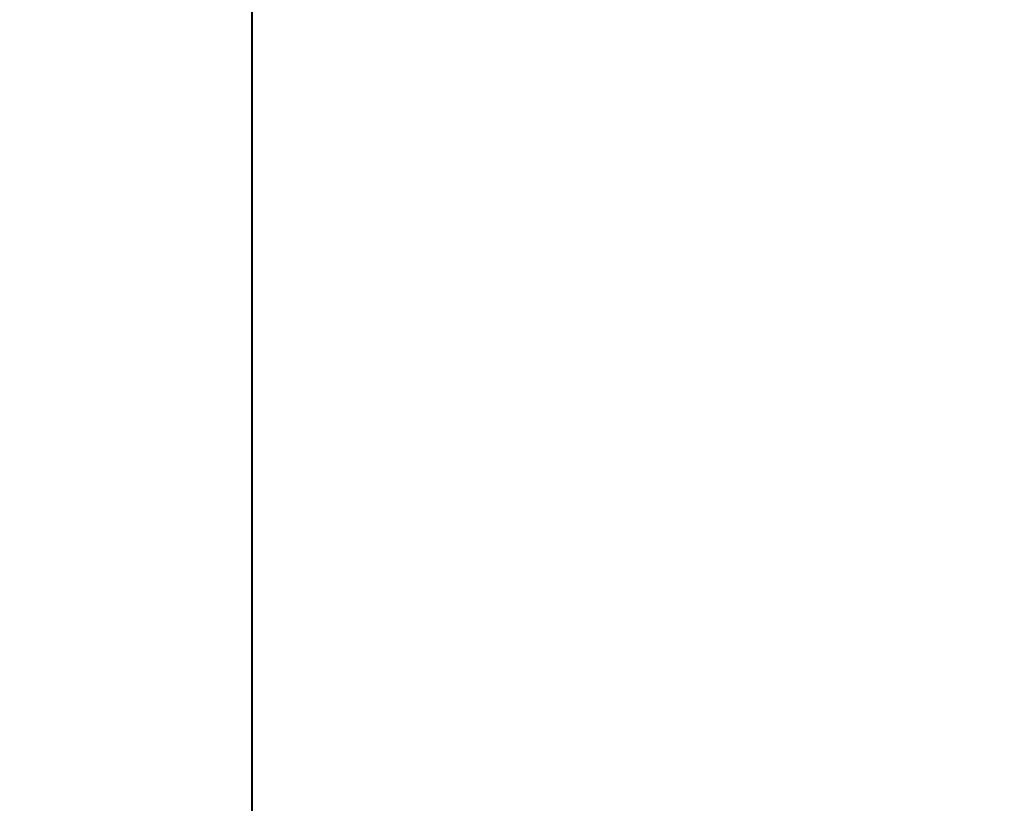
# Model space of a CAD drawing. Units: inches. Extents: x 459864 to 460310, y 324185 to 324787.
# Tile 99 of 112: x 460246.614 to 460248.739, y 324285.121 to 324286.812. Entities that reach past the tile are written whole.
import ezdxf

# ---------------------------------------------------------------- set-up
doc = ezdxf.new("R2010")
doc.units = ezdxf.units.IN
doc.layers.add('A-ANNO-DIMS', color=2, linetype='Continuous', lineweight=18)
doc.layers.add('A-WALL', color=7, linetype='Continuous', lineweight=40)
doc.styles.get("Standard").update_dxf_attribs({"font": 'arial.ttf'})
doc.dimstyles.new('ISO-25', dxfattribs={"dimtxt": 6, "dimasz": 2.5, "dimexe": 1.25, "dimexo": 0.625, "dimtad": 1, "dimdec": 1, "dimlunit": 3, "dimtxsty": 'Standard', "dimcen": 2.5, "dimadec": 0, "dimazin": 0, "dimtfac": 1, "dimtdec": 1, "dimtmove": 0, "dimatfit": 3, "dimfxl": 1, "dimarcsym": 0})

# ---------------------------------------------------------------- blocks, each defined once
blk = doc.blocks.new('*D21')
at = {"layer": 'A-ANNO-DIMS', "color": 0, "lineweight": -2, "transparency": 16777216}
for p, q in [((460247.7399, 324715.4832), (460309.5804, 324715.4832)), ((460308.3304, 324712.9832), (460308.3304, 324285.9832)), ((460247.7399, 324283.4832), (460309.5804, 324283.4832))]:
    blk.add_line(p, q, dxfattribs=at)
at = {"layer": 'A-ANNO-DIMS', "color": 0, "transparency": 16777216}
for points in [[(460307.9137, 324712.9832), (460308.747, 324712.9832), (460308.3304, 324715.4832)], [(460307.9137, 324285.9832), (460308.747, 324285.9832), (460308.3304, 324283.4832)]]:
    blk.add_solid(points, dxfattribs=at)
at = {"layer": 'Defpoints', "color": 0, "transparency": 16777216}
for p in [(460247.1149, 324715.4832), (460247.1149, 324283.4832), (460308.3304, 324283.4832)]:
    blk.add_point(p, dxfattribs=at)
at = {"layer": 'A-ANNO-DIMS', "color": 0, "transparency": 16777216, "insert": (460304.6399, 324499.4832), "char_height": 6, "attachment_point": 5, "rotation": 90}
blk.add_mtext("36'", dxfattribs=at)
blk = doc.blocks.new('*D62')
at = {"layer": 'A-ANNO-DIMS', "color": 0, "lineweight": -2, "transparency": 16777216}
for p, q in [((460247.7399, 324332.7387), (460278.7649, 324332.7387)), ((460277.5149, 324330.2387), (460277.5149, 324285.9832)), ((460247.7399, 324283.4832), (460278.7649, 324283.4832))]:
    blk.add_line(p, q, dxfattribs=at)
at = {"layer": 'A-ANNO-DIMS', "color": 0, "transparency": 16777216}
for points in [[(460277.0983, 324330.2387), (460277.9316, 324330.2387), (460277.5149, 324332.7387)], [(460277.0983, 324285.9832), (460277.9316, 324285.9832), (460277.5149, 324283.4832)]]:
    blk.add_solid(points, dxfattribs=at)
at = {"layer": 'Defpoints', "color": 0, "transparency": 16777216}
for p in [(460247.1149, 324332.7387), (460247.1149, 324283.4832), (460277.5149, 324283.4832)]:
    blk.add_point(p, dxfattribs=at)
at = {"layer": 'A-ANNO-DIMS', "color": 0, "transparency": 16777216, "insert": (460273.7876, 324308.111), "char_height": 6, "attachment_point": 5, "rotation": 90}
blk.add_mtext('4\'-1 1/2"', dxfattribs=at)
blk = doc.blocks.new('*D67')
at = {"layer": 'A-ANNO-DIMS', "color": 0, "lineweight": -2, "transparency": 16777216}
for p, q in [((460208.1149, 324284.1082), (460208.1149, 324315.1332)), ((460247.1149, 324284.1082), (460247.1149, 324315.1332)), ((460210.6149, 324313.8832), (460244.6149, 324313.8832))]:
    blk.add_line(p, q, dxfattribs=at)
at = {"layer": 'A-ANNO-DIMS', "color": 0, "transparency": 16777216}
for points in [[(460210.6149, 324314.2999), (460210.6149, 324313.4666), (460208.1149, 324313.8832)], [(460244.6149, 324314.2999), (460244.6149, 324313.4666), (460247.1149, 324313.8832)]]:
    blk.add_solid(points, dxfattribs=at)
at = {"layer": 'Defpoints', "color": 0, "transparency": 16777216}
for p in [(460247.1149, 324313.8832), (460208.1149, 324283.4832), (460247.1149, 324283.4832)]:
    blk.add_point(p, dxfattribs=at)
at = {"layer": 'A-ANNO-DIMS', "color": 0, "transparency": 16777216, "insert": (460227.6149, 324317.5737), "char_height": 6, "attachment_point": 5}
blk.add_mtext('3\'-3"', dxfattribs=at)

msp = doc.modelspace()

# ---------------------------------------------------------------- linework, layer by layer
at = {"layer": 'A-WALL'}
msp.add_line((460247.1149, 324470.9832), (460247.1149, 324283.4832), dxfattribs=at)

# ---------------------------------------------------------------- dimensions: what is measured, and where the dimension line sits
at = {"layer": 'A-ANNO-DIMS'}
for base, p1, angle, override, picture, middle in [((460308.3304, 324283.4832), (460247.1149, 324715.4832), 90, {"dimclrd": 0, "dimclre": 0, "dimclrt": 0}, '*D21', (460304.6399, 324499.4832)), ((460277.5149, 324283.4832), (460247.1149, 324332.7387), 270, {"dimdec": 1, "dimlfac": 1, "dimrnd": 0, "dimzin": 1, "dimdsep": 46, "dimlunit": 4, "dimfrac": 2}, '*D62', (460273.7876, 324308.111))]:
    dim = msp.add_linear_dim(base=base, p1=p1, p2=(460247.1149, 324283.4832), angle=angle, dimstyle='ISO-25', override=override, dxfattribs=at)
    dim.commit()
    dim.dimension.update_dxf_attribs({"geometry": picture, "text_midpoint": middle})
dim = msp.add_linear_dim(base=(460247.1149, 324313.8832), p1=(460208.1149, 324283.4832), p2=(460247.1149, 324283.4832), dimstyle='ISO-25', override={"dimdec": 1, "dimlfac": 1, "dimrnd": 0, "dimzin": 1, "dimdsep": 46, "dimlunit": 4, "dimfrac": 2}, dxfattribs=at)
dim.commit()
dim.dimension.update_dxf_attribs({"geometry": '*D67', "text_midpoint": (460227.6149, 324317.5737)})

doc.saveas('drawing.dxf')
